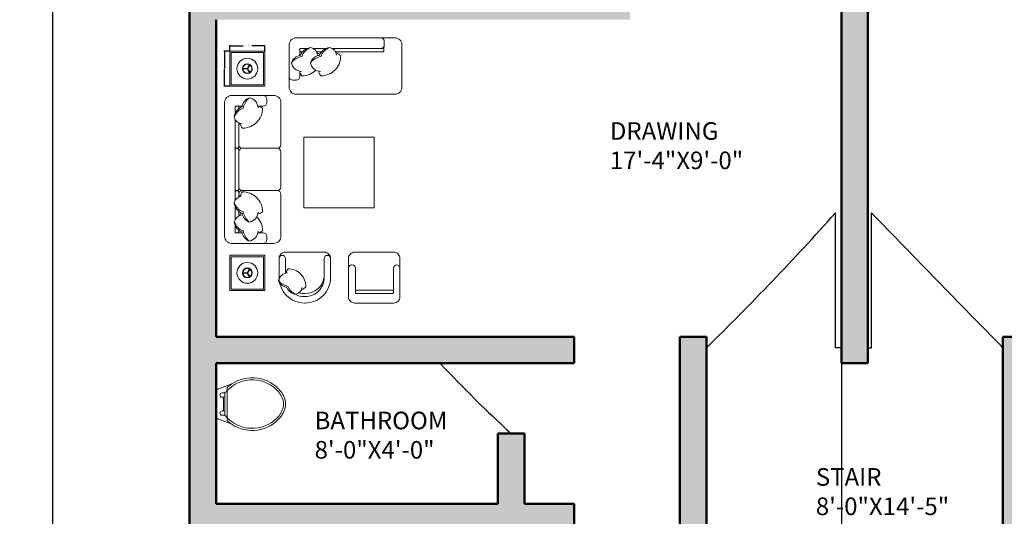
# Model space of a CAD drawing. Units: inches. Extents: x -17 to 536, y -817 to 53.
# Tile 2 of 9: x -17 to 319, y -606 to -436. Entities that reach past the tile are written whole.
import ezdxf

# ---------------------------------------------------------------- set-up
doc = ezdxf.new("R2010")
doc.units = ezdxf.units.IN
doc.header["$MEASUREMENT"] = 0
for name, color, linetype, lineweight in [('A-ANNO-DIMS', 2, 'Continuous', 18), ('A-AREA-IDEN', 7, 'Continuous', 18), ('A-DOOR', 4, 'Continuous', 25), ('A-FLOR-FIXT', 9, 'Continuous', 18), ('A-FURN', 8, 'Continuous', 13), ('A-WALL', 7, 'Continuous', 50), ('A-WALL-PATT', 22, 'Continuous', 13)]:
    doc.layers.add(name, color=color, linetype=linetype, lineweight=lineweight)
doc.styles.get("Standard").update_dxf_attribs({"font": 'arial.ttf'})
doc.dimstyles.get("Standard").update_dxf_attribs({"dimtxt": 0.18, "dimasz": 0.18, "dimexe": 0.18, "dimexo": 0.0625, "dimgap": 0.09, "dimtad": 0, "dimtih": 1, "dimtoh": 1, "dimdec": 0, "dimzin": 0, "dimdsep": 46, "dimlunit": 3, "dimtxsty": 'Standard', "dimcen": 0.09, "dimadec": 0, "dimazin": 0, "dimtfac": 1, "dimtdec": 0, "dimtofl": 0, "dimtmove": 0, "dimatfit": 3, "dimfxl": 1, "dimtolj": 1, "dimtzin": 0, "dimarcsym": 0})

# ---------------------------------------------------------------- blocks, each defined once
blk = doc.blocks.new('*D2')
at = {"layer": 'A-ANNO-DIMS', "color": 0, "lineweight": -2, "transparency": 16777216}
for p, q in [((41.3, 11.55), (-5.38, 11.55)), ((-5.2, 11.37), (-5.2, -378.8)), ((-5.2, -775.27), (-5.2, -385.1)), ((41.3, -775.45), (-5.38, -775.45))]:
    blk.add_line(p, q, dxfattribs=at)
at = {"layer": 'A-ANNO-DIMS', "color": 0, "transparency": 16777216}
for points in [[(-5.23, 11.37), (-5.17, 11.37), (-5.2, 11.55)], [(-5.23, -775.27), (-5.17, -775.27), (-5.2, -775.45)]]:
    blk.add_solid(points, dxfattribs=at)
at = {"layer": 'Defpoints', "color": 0, "transparency": 16777216}
for p in [(41.37, 11.55), (-5.2, -775.45), (41.37, -775.45)]:
    blk.add_point(p, dxfattribs=at)
at = {"layer": 'A-ANNO-DIMS', "color": 0, "transparency": 16777216, "insert": (-5.2, -381.95), "char_height": 6, "attachment_point": 5}
blk.add_mtext('\\A1;65\'-7"', dxfattribs=at)
blk = doc.blocks.new('DAY BED1')
at = {"color": 0}
blk.add_line((0.3, 0.25), (0.225, 0.255), dxfattribs=at)
blk.add_lwpolyline([(-0.3, 0, -0.414214), (-0.4, 0.1), (-0.4, 0.1, 0.317837), (-0.4, 0.1, -0.414214), (-0.4, 0.1), (-0.4, 0.1, 1.186185), (-0.4, 0.1, -0.414214), (-0.4, 0.1), (-0.4, 1.5, -0.414214), (-0.3, 1.6), (0.3, 1.6, -0.414214), (0.4, 1.5), (0.4, 0.1, -0.414214), (0.3, 0)], format="xyb", close=True, dxfattribs=at)
for points in [[(-0.073, 1.45), (-0.15, 1.45, -0.414214), (-0.2, 1.5), (-0.2, 1.55, -0.414214), (-0.15, 1.6)], [(-0.076, 1.425, -0.356772), (0.05, 1.568, -0.249542), (0.154, 1.438, 9.61688)], [(0.05, 1.568, -0.14773), (0.136, 1.422, -0.213343), (0.262, 1.293, -0.178662)], [(-0.073, 1.45, 0.165541), (-0.139, 1.419, 0.200231), (-0.058, 1.221, 0.121523)], [(0.143, 1.442, -0.306663), (0.262, 1.293, -0.30633), (0.154, 1.196, 0.872847)], [(0.25, 1.345), (0.25, 1.45), (0.152, 1.45, -0.414214)], [(0.2, 1.412), (0.2, 1.43, -0.414214), (0.22, 1.45), (0.23, 1.45, -0.414214), (0.25, 1.43)], [(0.25, 1.43), (0.25, 1.345, -0.414214)], [(-0.076, 1.156, -0.356772), (0.05, 1.299, -0.249542), (0.154, 1.169, 9.61688)], [(0.05, 1.299, -0.14773), (0.136, 1.153, -0.213343), (0.262, 1.024, -0.178662)], [(0.25, 1.262), (0.25, 1.075, -0.414214)], [(-0.073, 1.181, 0.165541), (-0.139, 1.15, 0.425989), (0.148, 0.869, 0.121523), (0.187, 0.936, -7.115464)], [(0.143, 1.173, -0.306663), (0.262, 1.024, -0.30633), (0.154, 0.926, 0.872847)], [(0.168, 1.163, 0.071865), (0.187, 1.205, -7.115464)], [(0.2, 1.142), (0.2, 1.211, -0.414214)], [(0.25, 0.992), (0.25, 0.275, -0.414214), (0.23, 0.255), (0.22, 0.255, -0.414214), (0.2, 0.275), (0.2, 0.942, -0.414214)], [(0.25, 0.377), (0.25, 0.3, 0.414214), (0.3, 0.25), (0.35, 0.25, 0.414214), (0.4, 0.3)]]:
    blk.add_lwpolyline(points, format="xyb", dxfattribs=at)
for points in [[(0.25, 1.075), (0.25, 1.262)], [(0.25, 0.377), (0.25, 0.992)]]:
    blk.add_lwpolyline(points, dxfattribs=at)
blk = doc.blocks.new('WC-23IN')
for p, q in [((3.55, 13.58), (3.55, 14.57)), ((3.55, 13.58), (3.55, 8.97)), ((3.55, 4.35), (3.55, 8.97)), ((3.55, 3.36), (3.55, 4.35))]:
    blk.add_line(p, q)
for points in [[(3.55, 13.58, -0.448546), (21.24, 12.93, -0.162618), (22.76, 8.97, -0.470877)], [(5.16, 15.84, -0.383919), (21.78, 13.38, -0.163732), (23.47, 8.97, -0.359733)], [(0, 8.97), (0, 13.45, -0.31031), (0.38, 14), (5.16, 15.84, -0.209071)], [(2.84, 12.77, -0.022712), (3.55, 13.58, -0.162618)], [(3.55, 14.57, -0.040937), (5.16, 15.84, -0.163732)], [(2.84, 12.77), (1.86, 12.77, 1), (1.86, 11.28), (2.37, 11.28)], [(2.84, 8.97), (2.84, 12.77, -0.476108)], [(0, 8.97), (0, 4.48, 0.31031), (0.38, 3.94), (5.16, 2.09, 0.209071)], [(2.84, 8.97), (2.84, 5.16, 0.022712)], [(4.03, 3.88, 0.431639), (21.24, 5, 0.162618), (22.76, 8.97, 0.470877)], [(5.16, 2.09, 0.383919), (21.78, 4.55, 0.163732), (23.47, 8.97, 0.359733)], [(2.84, 5.16), (1.86, 5.16, -1), (1.86, 6.66), (2.37, 6.66)], [(2.84, 5.16, 0.022712), (3.55, 4.35, 0.162618)], [(3.55, 4.35, 0.014165), (4.03, 3.88, 0.162618)], [(3.55, 3.36, 0.040937), (5.16, 2.09, 0.163732)]]:
    blk.add_lwpolyline(points, format="xyb")
for points in [[(2.37, 11.28), (2.37, 6.66)], [(2.37, 11.28), (2.84, 11.28)], [(2.37, 6.66), (2.84, 6.66)]]:
    blk.add_lwpolyline(points)
blk = doc.blocks.new('END-TABLE-LAMP-A')
for p, q in [((5.93, 6.04), (6.78, 7.5)), ((6.06, 5.96), (6.91, 7.43)), ((6, 6.07), (4.31, 6.07)), ((6, 5.92), (4.31, 5.92)), ((5.93, 5.96), (6.78, 4.5)), ((6.06, 6.04), (6.91, 4.57))]:
    blk.add_line(p, q)
at = {"ltscale": 0.03}
blk.add_lwpolyline([(12, 12), (12, 0), (0, 0), (0, 12)], close=True, dxfattribs=at)
blk.add_lwpolyline([(11.52, 0.48), (11.52, 11.52), (0.48, 11.52), (0.48, 0.48)], close=True)
for radius in [3.54, 1.69, 1.52]:
    blk.add_circle((6, 6), radius)
blk = doc.blocks.new('*D32')
at = {"layer": 'A-ANNO-DIMS', "color": 0, "lineweight": -2, "transparency": 16777216}
for p, q in [((55.03, -447.08), (55.03, -445.16)), ((55.21, -445.34), (59.55, -445.34)), ((66.85, -445.34), (62.52, -445.34)), ((67.03, -447.08), (67.03, -445.16))]:
    blk.add_line(p, q, dxfattribs=at)
at = {"layer": 'A-ANNO-DIMS', "color": 0, "transparency": 16777216}
for points in [[(55.21, -445.31), (55.21, -445.37), (55.03, -445.34)], [(66.85, -445.31), (66.85, -445.37), (67.03, -445.34)]]:
    blk.add_solid(points, dxfattribs=at)
at = {"layer": 'Defpoints', "color": 0, "transparency": 16777216}
for p in [(67.03, -445.34), (55.03, -447.14), (67.03, -447.14)]:
    blk.add_point(p, dxfattribs=at)
at = {"layer": 'A-ANNO-DIMS', "color": 0, "transparency": 16777216, "insert": (61.03, -445.34), "char_height": 0.18, "attachment_point": 5}
blk.add_mtext('\\A1;END TABLE A 1\'-0" TYP.', dxfattribs=at)
blk = doc.blocks.new('*D33')
at = {"layer": 'A-ANNO-DIMS', "color": 0, "lineweight": -2, "transparency": 16777216}
for p, q in [((54.97, -447.14), (53.05, -447.14)), ((53.23, -447.32), (53.23, -452.96)), ((53.23, -458.96), (53.23, -453.32)), ((54.97, -459.14), (53.05, -459.14))]:
    blk.add_line(p, q, dxfattribs=at)
at = {"layer": 'A-ANNO-DIMS', "color": 0, "transparency": 16777216}
for points in [[(53.2, -447.32), (53.26, -447.32), (53.23, -447.14)], [(53.2, -458.96), (53.26, -458.96), (53.23, -459.14)]]:
    blk.add_solid(points, dxfattribs=at)
at = {"layer": 'Defpoints', "color": 0, "transparency": 16777216}
for p in [(53.23, -447.14), (55.03, -447.14), (55.03, -459.14)]:
    blk.add_point(p, dxfattribs=at)
at = {"layer": 'A-ANNO-DIMS', "color": 0, "transparency": 16777216, "insert": (53.23, -453.14), "char_height": 0.18, "attachment_point": 5}
blk.add_mtext('\\A1;1\'-0" TYP.', dxfattribs=at)
blk = doc.blocks.new('*D40')
at = {"layer": 'A-ANNO-DIMS', "color": 0, "lineweight": -2, "transparency": 16777216}
for p, q in [((217.37, -544.51), (217.37, -816.98)), ((263.37, -553.51), (263.37, -816.98)), ((217.55, -816.8), (239.97, -816.8)), ((263.19, -816.8), (240.76, -816.8))]:
    blk.add_line(p, q, dxfattribs=at)
at = {"layer": 'A-ANNO-DIMS', "color": 0, "transparency": 16777216}
for points in [[(217.55, -816.77), (217.55, -816.83), (217.37, -816.8)], [(263.19, -816.77), (263.19, -816.83), (263.37, -816.8)]]:
    blk.add_solid(points, dxfattribs=at)
at = {"layer": 'Defpoints', "color": 0, "transparency": 16777216}
for p in [(217.37, -544.45), (263.37, -553.45), (263.37, -816.8)]:
    blk.add_point(p, dxfattribs=at)
at = {"layer": 'A-ANNO-DIMS', "color": 0, "transparency": 16777216, "insert": (240.37, -816.8), "char_height": 0.18, "attachment_point": 5}
blk.add_mtext('\\A1;3\'-10"', dxfattribs=at)

msp = doc.modelspace()

# ---------------------------------------------------------------- hatches: boundary and pattern name
at = {"layer": 'A-WALL-PATT'}
h = msp.add_hatch(color=256, dxfattribs=at)
h.dxf.hatch_style = 1
h.paths.add_polyline_path([(217.37, -544.45), (208.37, -544.45), (208.37, -775.45), (217.37, -775.45)], flags=17)
h.paths.add_polyline_path([(327.37, -544.45), (318.37, -544.45), (318.37, -775.45), (327.37, -775.45)], flags=17)
h.paths.add_polyline_path([(494.37, 11.55), (41.37, 11.55), (41.37, -775.45), (50.37, -775.45), (50.37, -739.45), (184.37, -739.45), (184.37, -730.45), (50.37, -730.45), (50.37, -610.45), (172.37, -610.45), (172.37, -601.45), (155.37, -601.45), (155.37, -577.45), (146.37, -577.45), (146.37, -601.45), (50.37, -601.45), (50.37, -553.45), (172.37, -553.45), (172.37, -544.45), (50.37, -544.45), (50.37, -436.45), (191.37, -436.45), (191.37, -319.45), (182.37, -319.45), (182.37, -427.45), (50.37, -427.45), (50.37, -283.45), (98.37, -283.45), (98.37, -274.45), (50.37, -274.45), (50.37, -219.45), (122.37, -219.45), (122.37, -283.45), (191.37, -283.45), (191.37, -274.45), (131.37, -274.45), (131.37, -219.45), (131.37, -150.45), (146.37, -150.45), (146.37, -141.45), (122.37, -141.45), (122.37, -210.45), (50.37, -210.45), (50.37, -150.45), (98.37, -150.45), (98.37, -141.45), (50.37, -141.45), (50.37, 2.55), (182.37, 2.55), (182.37, -150.45), (191.37, -150.45), (191.37, 2.55), (263.37, 2.55), (263.37, -141.45), (227.37, -141.45), (227.37, -150.45), (263.37, -150.45), (263.37, -553.45), (272.37, -553.45), (272.37, -150.45), (308.37, -150.45), (308.37, -141.45), (272.37, -141.45), (272.37, 2.55), (344.37, 2.55), (344.37, -150.45), (353.37, -150.45), (353.37, 2.55), (485.37, 2.55), (485.37, -141.45), (437.37, -141.45), (437.37, -150.45), (485.37, -150.45), (485.37, -210.45), (413.37, -210.45), (413.37, -141.45), (389.37, -141.45), (389.37, -150.45), (404.37, -150.45), (404.37, -219.45), (404.37, -274.45), (353.37, -274.45), (344.37, -274.45), (344.37, -283.45), (353.37, -283.45), (413.37, -283.45), (413.37, -219.45), (485.37, -219.45), (485.37, -274.45), (437.37, -274.45), (437.37, -283.45), (485.37, -283.45), (485.37, -427.45), (353.37, -427.45), (353.37, -319.45), (344.37, -319.45), (344.37, -436.45), (485.37, -436.45), (485.37, -544.45), (363.37, -544.45), (363.37, -553.45), (485.37, -553.45), (485.37, -601.45), (389.37, -601.45), (389.37, -577.45), (380.37, -577.45), (380.37, -601.45), (363.37, -601.45), (363.37, -610.45), (485.37, -610.45), (485.37, -730.45), (351.37, -730.45), (351.37, -739.45), (485.37, -739.45), (485.37, -775.45), (494.37, -775.45)])

# ---------------------------------------------------------------- linework, layer by layer
at = {"layer": 'A-DOOR'}
for p, q in [((261.36, -512.24), (261.36, -502.24)), ((273.58, -512.24), (273.58, -502.24)), ((261.36, -548.24), (261.36, -512.24)), ((273.58, -548.24), (273.58, -512.24)), ((263.37, -548.24), (261.36, -548.24)), ((272.37, -548.24), (273.58, -548.24)), ((150.87, -553.7), (126.87, -553.7)), ((150.87, -553.7), (150.87, -553.45))]:
    msp.add_line(p, q, dxfattribs=at)
for centre, radius, start, end in [((-452.11, 136.05), 957.31, 314.37297, 318.18316), ((6994.85, 5997.03), 9349.65, 224.03799, 224.431428), ((463.84, -237.15), 462.35, 223.2102, 227.3952)]:
    msp.add_arc(centre, radius, start, end, dxfattribs=at)
at = {"layer": 'A-FURN', "ltscale": 0.03}
for points in [[(70.06, -462.29, -0.414214), (72.46, -464.69), (72.46, -479.08, -0.414214), (71.26, -480.28, -0.414214), (72.46, -481.48), (72.46, -493.48, -0.414214), (71.26, -494.68, -0.414214), (72.46, -495.88), (72.46, -510.28, -0.414214), (70.06, -512.68), (55.67, -512.68, -0.414214), (53.27, -510.28), (53.27, -464.69, -0.414214), (55.67, -462.29)], [(110.83, -532.98), (110.83, -532.98, 0.414214), (112.99, -530.81), (112.99, -517.83, 0.414214), (110.83, -515.67), (110.83, -515.67), (97.63, -515.67, 0.414214), (95.47, -517.83), (95.47, -530.81, 0.414214), (97.63, -532.98)]]:
    msp.add_lwpolyline(points, format="xyb", close=True, dxfattribs=at)
at = {"layer": 'A-FURN'}
for points in [[(66.46, -462.29, -0.414214), (67.66, -463.49), (67.66, -464.69, -0.414214), (66.46, -465.89), (64.61, -465.89)], [(61.65, -463.05, 0.14773), (59.59, -466.56, 0.213343), (56.57, -469.65, 0.178662)], [(59.43, -466.07, 0.306663), (56.57, -469.65, 0.30633), (59.18, -471.99, -0.872847)], [(58.07, -466.8), (58.07, -466.37, 0.414214), (57.59, -465.89), (57.35, -465.89, 0.414214), (56.87, -466.37)], [(64.61, -465.89, -0.165541), (66.19, -466.63, -0.425989), (59.32, -473.37, -0.121523), (58.37, -471.77, 7.115464)], [(64.68, -466.49, 0.356772), (61.65, -463.05, 0.249542), (59.16, -466.17, -9.61688)], [(56.87, -466.37), (56.87, -468.41, 0.414214)], [(56.87, -470.41), (56.87, -479.8, 0.414214), (57.35, -480.28), (57.59, -480.28, 0.414214), (58.07, -479.8), (58.07, -471.62, 0.414214)], [(58.07, -479.08, 0.414214), (59.27, -480.28), (71.26, -480.28, 0.414214)], [(58.07, -481.48, -0.414214), (59.27, -480.28)], [(56.87, -498.1), (56.87, -495.16, -0.414214), (57.35, -494.68), (57.59, -494.68, -0.414214), (58.07, -495.16), (58.07, -496.89, -0.414214)], [(58.07, -493.48, 0.414214), (59.27, -494.68)], [(58.07, -495.88, -0.414214), (59.27, -494.68), (71.26, -494.68, -0.414214)], [(64.61, -502.62, 0.165541), (66.19, -501.88, 0.425989), (59.32, -495.14, 0.121523), (58.37, -496.74, -7.115464)], [(59.43, -502.43, -0.306663), (56.57, -498.85, -0.30633), (59.18, -496.51, 0.872847)], [(61.65, -505.45, -0.14773), (59.59, -501.94, -0.213343), (56.57, -498.85, -0.178662)], [(59.43, -508.89, -0.306663), (56.57, -505.31, -0.30633), (59.18, -502.98, 0.872847)], [(56.87, -504.56), (56.87, -500.09, -0.414214)], [(58.07, -501.7), (58.07, -503.35, -0.414214)], [(58.84, -502.19, 0.071865), (58.37, -503.2, -7.115464)], [(64.68, -502.01, -0.356772), (61.65, -505.45, -0.249542), (59.16, -502.34, 9.61688)], [(61.65, -511.91, -0.14773), (59.59, -508.41, -0.213343), (56.57, -505.31, -0.178662)], [(64.61, -509.08, 0.165541), (66.19, -508.34, 0.200231), (64.26, -503.58, 0.121523)], [(56.87, -506.55), (56.87, -509.08), (59.22, -509.08, -0.414214)], [(56.87, -508.6), (56.87, -506.55, -0.414214)], [(58.07, -508.16), (58.07, -508.6, -0.414214), (57.59, -509.08), (57.35, -509.08, -0.414214), (56.87, -508.6)], [(64.68, -508.48, -0.356772), (61.65, -511.91, -0.249542), (59.16, -508.8, 9.61688)], [(64.61, -509.08), (66.46, -509.08, -0.414214), (67.66, -510.28), (67.66, -511.48, -0.414214), (66.46, -512.68)], [(73.99, -522.81), (73.99, -517.83, 0.414214), (72.91, -516.75), (72.91, -516.75, 0.414214), (71.83, -517.83)], [(87.19, -524.32), (87.19, -517.83, -0.414214), (88.27, -516.75), (88.27, -516.75, -0.414214), (89.35, -517.83)], [(74.75, -522.69, 0.356772), (71.65, -525.42, 0.249542), (74.46, -527.66, -9.61688)], [(74.2, -522.75, -0.165541), (74.87, -521.33, -0.425989), (80.95, -527.52, -0.121523), (79.51, -528.38, 7.115464)], [(95.47, -521.08, -0.414214), (96.55, -520), (96.76, -520, -0.414214), (97.85, -521.08), (97.85, -522.75)], [(110.83, -529.08), (110.83, -521.08, -0.414214), (111.91, -520), (111.91, -520, -0.414214), (112.99, -521.08)], [(71.65, -525.42, 0.14773), (74.81, -527.27, 0.213343), (77.6, -530, 0.178662)], [(87.19, -524.32, -0.372719), (80.7, -529.73), (80.59, -529.73)], [(87.19, -524.32, -0.414214), (80.7, -530.81), (80.59, -530.81)], [(74.37, -527.42, 0.306663), (77.6, -530, 0.30633), (79.71, -527.65, -0.872847)], [(78.64, -529.5, 0.072384), (80.48, -529.73), (80.59, -529.73)], [(103.01, -528.65), (98.28, -528.65, 0.414214), (97.85, -529.08), (97.85, -529.3, 0.414214), (98.28, -529.73)], [(98.28, -529.73), (101.92, -529.73, 0.414214)], [(101.92, -529.73), (110.39, -529.73, 0.414214), (110.83, -529.3), (110.83, -529.08, 0.414214), (110.39, -528.65), (103.01, -528.65, 0.414214)], [(77.26, -529.96, 0.130591), (80.48, -530.81), (80.59, -530.81)]]:
    msp.add_lwpolyline(points, format="xyb", dxfattribs=at)
for points in [[(59.22, -465.89), (56.87, -465.89), (56.87, -468.41)], [(56.87, -470.41), (56.87, -498.1)], [(56.87, -500.09), (56.87, -504.56)], [(97.85, -522.75), (97.85, -529.73), (101.92, -529.73)], [(101.92, -529.73), (110.72, -529.73)]]:
    msp.add_lwpolyline(points, dxfattribs=at)
at = {"layer": 'A-FURN', "ltscale": 0.03}
msp.add_lwpolyline([(104.22, -500.53), (104.22, -476.53), (80.23, -476.53), (80.23, -500.53)], close=True, dxfattribs=at)
at = {"layer": 'A-FURN'}
msp.add_lwpolyline([(56.87, -494.2), (56.87, -480.76, -0.414214), (57.35, -480.28), (57.59, -480.28, -0.414214), (58.07, -480.76), (58.07, -494.2, -0.414214), (57.59, -494.68), (57.35, -494.68, -0.414214)], format="xyb", close=True, dxfattribs=at)
at = {"layer": 'A-FURN', "ltscale": 0.03}
msp.add_lwpolyline([(80.59, -515.67), (87.19, -515.67, -0.414214), (89.35, -517.83), (89.35, -524.32, -0.414214), (80.7, -532.98), (80.59, -532.98), (80.48, -532.98, -0.414214), (71.83, -524.32), (71.83, -517.83, -0.414214), (73.99, -515.67), (80.59, -515.67)], format="xyb", dxfattribs=at)
at = {"layer": 'A-WALL'}
for p, q in [((41.37, 11.55), (41.37, -775.45)), ((263.37, -150.45), (263.37, -553.45)), ((272.37, -150.45), (272.37, -553.45)), ((50.37, -436.45), (50.37, -544.45)), ((50.37, -544.45), (172.37, -544.45)), ((172.37, -553.45), (172.37, -544.45)), ((208.37, -544.45), (208.37, -775.45)), ((208.37, -544.45), (217.37, -544.45)), ((217.37, -544.45), (217.37, -775.45)), ((318.37, -544.45), (318.37, -775.45)), ((318.37, -544.45), (327.37, -544.45)), ((50.37, -553.45), (172.37, -553.45)), ((50.37, -553.45), (50.37, -601.45)), ((263.37, -553.45), (272.37, -553.45)), ((146.37, -577.45), (146.37, -601.45)), ((146.37, -577.45), (155.37, -577.45)), ((155.37, -577.45), (155.37, -601.45)), ((50.37, -601.45), (146.37, -601.45)), ((155.37, -601.45), (172.37, -601.45)), ((172.37, -601.45), (172.37, -610.45))]:
    msp.add_line(p, q, dxfattribs=at)

# ---------------------------------------------------------------- block references
at = {"layer": 'A-FLOR-FIXT'}
msp.add_blockref('WC-23IN', (50.57, -576.38), dxfattribs=at)
at = {"layer": 'A-FURN', "ltscale": 0.03, "xscale": 23.99467061322209, "yscale": 23.99467061322209, "zscale": 23.99467061322209, "rotation": 90}
msp.add_blockref('DAY BED1', (113.66, -452.24), dxfattribs=at)
at = {"layer": 'A-FURN'}
for p in [(55.03, -459.14), (55.03, -528.72)]:
    msp.add_blockref('END-TABLE-LAMP-A', p, dxfattribs=at)

# ---------------------------------------------------------------- texts
at = {"layer": 'A-AREA-IDEN', "char_height": 6, "attachment_point": 1}
for s, insert in [('DRAWING\\P17\'-4"X9\'-0"', (184.49, -471.37)), ('BATHROOM\\P8\'-0"X4\'-0"', (83.93, -570)), ('STAIR\\P8\'-0"X14\'-5"', (254.64, -589.24))]:
    msp.add_mtext(s, dxfattribs=dict(at, insert=insert))

# ---------------------------------------------------------------- dimensions: what is measured, and where the dimension line sits
at = {"layer": 'A-ANNO-DIMS'}
dim = msp.add_linear_dim(base=(-5.2, -775.45), p1=(41.37, 11.55), p2=(41.37, -775.45), angle=90, dimstyle='Standard', override={"dimtxt": 6, "dimclrd": 0, "dimclre": 0, "dimclrt": 0}, dxfattribs=at)
dim.commit()
dim.dimension.update_dxf_attribs({"geometry": '*D2', "text_midpoint": (-5.2, -381.95)})
dim = msp.add_linear_dim(base=(67.03, -445.34), p1=(55.03, -447.14), p2=(67.03, -447.14), text='END TABLE A <> TYP.', dimstyle='Standard', override={"dimdec": 1, "dimlfac": 1, "dimrnd": 0, "dimzin": 1, "dimdsep": 46, "dimlunit": 4, "dimfrac": 2}, dxfattribs=at)
dim.commit()
dim.dimension.update_dxf_attribs({"geometry": '*D32', "text_midpoint": (61.03, -445.34)})
dim = msp.add_linear_dim(base=(53.23, -447.14), p1=(55.03, -459.14), p2=(55.03, -447.14), angle=90, text='<> TYP.', dimstyle='Standard', override={"dimdec": 1, "dimlfac": 1, "dimrnd": 0, "dimzin": 1, "dimdsep": 46, "dimlunit": 4, "dimfrac": 2}, dxfattribs=at)
dim.commit()
dim.dimension.update_dxf_attribs({"geometry": '*D33', "text_midpoint": (53.23, -453.14)})
dim = msp.add_linear_dim(base=(263.37, -816.8), p1=(217.37, -544.45), p2=(263.37, -553.45), dimstyle='Standard', override={"dimdec": 1, "dimlfac": 1, "dimrnd": 0, "dimzin": 1, "dimdsep": 46, "dimlunit": 4, "dimfrac": 2}, dxfattribs=at)
dim.commit()
dim.dimension.update_dxf_attribs({"geometry": '*D40', "text_midpoint": (240.37, -816.8)})

doc.saveas('drawing.dxf')
